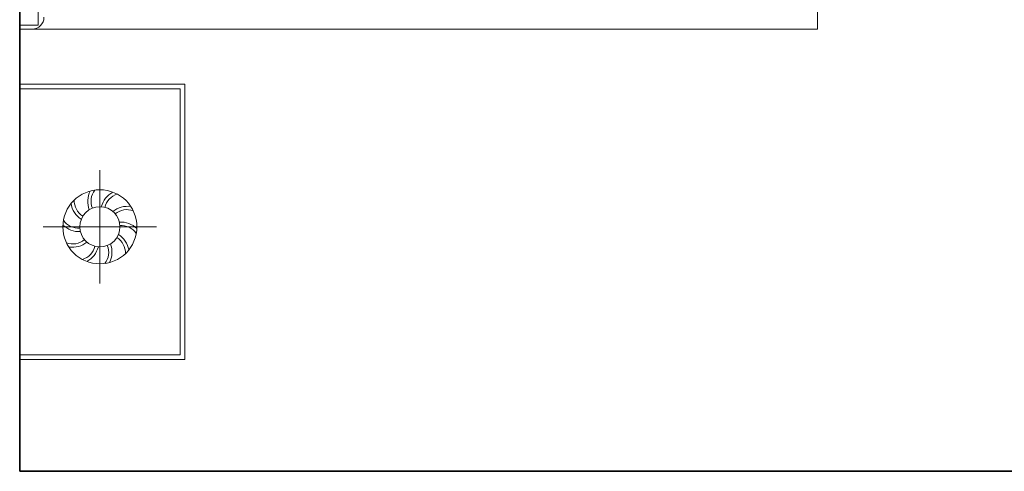
# Model space of a CAD drawing. Units: inches. Extents: x -638 to 186, y -762 to 59.
# Tile 5 of 31: x -161 to -100, y -539 to -511. Entities that reach past the tile are written whole.
import ezdxf

# ---------------------------------------------------------------- set-up
doc = ezdxf.new("R2010")
doc.units = ezdxf.units.IN
doc.layers.add('furn', color=8, linetype='Continuous', lineweight=13)
doc.layers.add('wall', color=7, linetype='Continuous', lineweight=35)

# ---------------------------------------------------------------- blocks, each defined once
blk = doc.blocks.new('BED-DOUBLE-WITH-NIGHTSTANDS')
for p, q in [((0, 59.951), (78.699, 59.951)), ((0, 49.874), (0, 59.951)), ((0.288, 50.162), (0.288, 59.951)), ((16.508, 59.951), (16.508, 50.162)), ((16.796, 59.951), (16.796, 49.874)), ((20.158, 59.951), (20.158, 11.244)), ((20.398, 58.826), (20.398, 59.951)), ((8.091, 51.596), (8.091, 58.516)), ((58.161, 58.826), (20.398, 58.826)), ((4.631, 55.056), (11.551, 55.056)), ((16.508, 50.162), (0.288, 50.162)), ((16.796, 49.874), (0, 49.874)), ((20.158, 11.244), (58.548, 11.244))]:
    blk.add_line(p, q)
for radius in [2.26, 1.225]:
    blk.add_circle((8.091, 55.056), radius)
for centre, radius, start, end in [((20.878, 59.188), 0.72, 180, 270), ((9.248, 56.308), 1.452, 136.17003, 182.48975), ((9.115, 56.366), 1.108, 124.30017, 184.53802), ((8.292, 56.749), 1.452, 172.17003, 218.48975), ((8.15, 56.718), 1.108, 160.30017, 220.53802), ((9.763, 55.389), 1.452, 100.17003, 146.48975), ((9.69, 55.514), 1.108, 88.30017, 148.53802), ((7.162, 56.435), 1.108, 196.30017, 256.53802), ((7.258, 56.544), 1.452, 208.17003, 254.48975), ((9.64, 54.343), 1.452, 64.17003, 110.48975), ((9.653, 54.487), 1.108, 52.30017, 112.53802), ((6.529, 55.625), 1.108, 232.30017, 292.53802), ((9.021, 53.678), 1.108, 16.30017, 76.53802), ((8.925, 53.569), 1.452, 28.17003, 74.48975), ((6.543, 55.77), 1.452, 244.17003, 290.48975), ((8.033, 53.395), 1.108, 340.30017, 40.53802), ((7.891, 53.363), 1.452, 352.17003, 38.48975), ((6.493, 54.599), 1.108, 268.30017, 328.53802), ((6.419, 54.723), 1.452, 280.17003, 326.48975), ((7.067, 53.747), 1.108, 304.30017, 4.53802), ((6.934, 53.804), 1.452, 316.17003, 2.48975)]:
    blk.add_arc(centre, radius, start, end)

msp = doc.modelspace()

# ---------------------------------------------------------------- linework, layer by layer
at = {"layer": 'wall'}
for p, q in [((-160.526, -412.533), (-160.526, -539.033)), ((-160.526, -539.033), (1.474, -539.033))]:
    msp.add_line(p, q, dxfattribs=at)

# ---------------------------------------------------------------- block references
at = {"layer": 'furn', "rotation": 90.00000000000017}
msp.add_blockref('BED-DOUBLE-WITH-NIGHTSTANDS', (-100.575, -532.203), dxfattribs=at)

doc.saveas('drawing.dxf')
